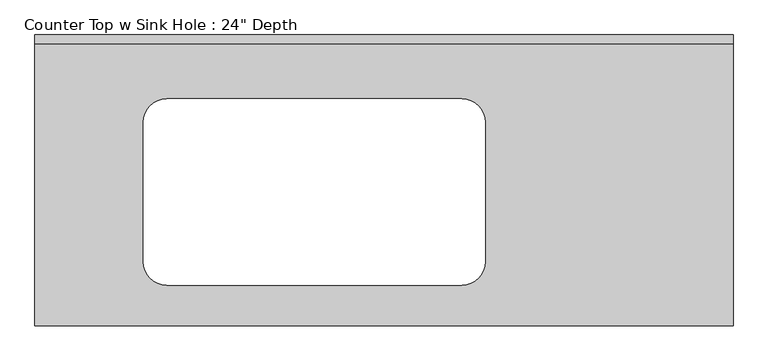
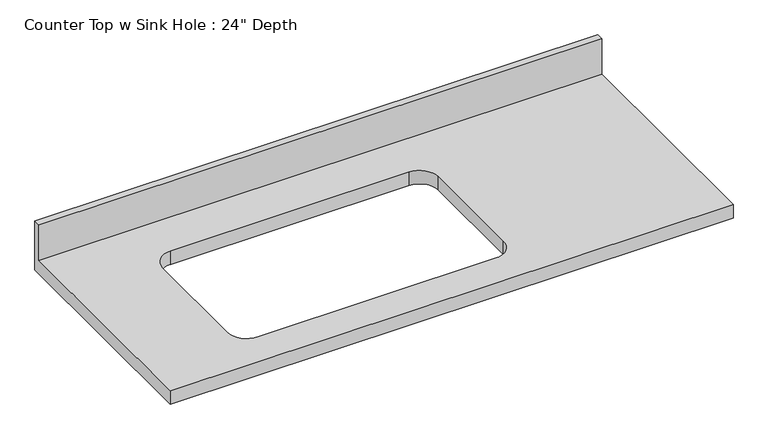
"""IFC4 building model written with IfcOpenShell, lengths in millimetres: furniture geometry."""

from ifc_helpers import new_model, si_unit, frame, origin, place, context, project, spatial, polyline, circle_curve, source, transform, mapped, element, save
from ifc_brep_helpers import plane_surface, revolved_surface, advanced_brep


def furniture_c9930e7d(model_context):
    return source(origin(), model_context, "Body", "AdvancedBrep", [
        advanced_brep(
        [(-1200.4622951, -635.0, 914.4), (323.5377049, -635.0, 914.4), (323.5377049, -19.05, 914.4), (-1200.4622951, -19.05, 914.4), (-913.0885418, -139.7, 914.4), (-268.6360484, -139.7, 914.4), (-217.8360484, -190.5, 914.4), (-217.8360484, -495.3, 914.4), (-268.6360484, -546.1, 914.4), (-913.0885418, -546.1, 914.4), (-963.8885418, -495.3, 914.4), (-963.8885418, -190.5, 914.4), (323.5377049, 0.0, 876.3), (323.5377049, -635.0, 876.3), (-1200.4622951, -635.0, 876.3), (-1200.4622951, 0.0, 876.3), (-268.6360484, -139.7, 876.3), (-913.0885418, -139.7, 876.3), (-963.8885418, -190.5, 876.3), (-963.8885418, -495.3, 876.3), (-913.0885418, -546.1, 876.3), (-268.6360484, -546.1, 876.3), (-217.8360484, -495.3, 876.3), (-217.8360484, -190.5, 876.3), (-1200.4622951, 0.0, 1016.0), (323.5377049, 0.0, 1016.0), (-1200.4622951, -19.05, 1016.0), (323.5377049, -19.05, 1016.0)],
        [
            (0, 1),
            (1, 2),
            (2, 3),
            (3, 0),
            (4, 5),
            (5, 6, circle_curve(frame((-268.6360484, -190.5, 914.4), z_axis=(0.0, 0.0, -1.0), x_axis=(1.0, 0.0, 0.0)), 50.8)),
            (6, 7),
            (7, 8, circle_curve(frame((-268.6360484, -495.3, 914.4), z_axis=(0.0, 0.0, -1.0), x_axis=(1.0, 0.0, 0.0)), 50.8)),
            (8, 9),
            (9, 10, circle_curve(frame((-913.0885418, -495.3, 914.4), z_axis=(0.0, 0.0, -1.0), x_axis=(1.0, 0.0, 0.0)), 50.8)),
            (10, 11),
            (11, 4, circle_curve(frame((-913.0885418, -190.5, 914.4), z_axis=(0.0, 0.0, -1.0), x_axis=(1.0, 0.0, 0.0)), 50.8)),
            (12, 13),
            (13, 14),
            (14, 15),
            (15, 12),
            (16, 17),
            (17, 18, circle_curve(frame((-913.0885418, -190.5, 876.3), z_axis=(0.0, 0.0, 1.0), x_axis=(1.0, 0.0, 0.0)), 50.8)),
            (18, 19),
            (19, 20, circle_curve(frame((-913.0885418, -495.3, 876.3), z_axis=(0.0, 0.0, 1.0), x_axis=(1.0, 0.0, 0.0)), 50.8)),
            (20, 21),
            (21, 22, circle_curve(frame((-268.6360484, -495.3, 876.3), z_axis=(0.0, 0.0, 1.0), x_axis=(1.0, 0.0, 0.0)), 50.8)),
            (22, 23),
            (23, 16, circle_curve(frame((-268.6360484, -190.5, 876.3), z_axis=(0.0, 0.0, 1.0), x_axis=(1.0, 0.0, 0.0)), 50.8)),
            (15, 24),
            (24, 25),
            (25, 12),
            (14, 0),
            (3, 26),
            (26, 24),
            (13, 1),
            (25, 27),
            (27, 2),
            (4, 17),
            (16, 5),
            (11, 18),
            (10, 19),
            (9, 20),
            (8, 21),
            (7, 22),
            (6, 23),
            (26, 27),
        ],
        [
            plane_surface(frame((-1200.4622951, 0.0, 914.4), z_axis=(0.0, 0.0, 1.0), x_axis=(-1.0, 0.0, 0.0))),
            plane_surface(frame((-1200.4622951, 0.0, 876.3), z_axis=(0.0, 0.0, -1.0), x_axis=(1.0, 0.0, 0.0))),
            plane_surface(frame((323.5377049, 0.0, 914.4), z_axis=(0.0, 1.0, 0.0), x_axis=(0.0, 0.0, -1.0))),
            plane_surface(frame((-1200.4622951, 0.0, 914.4), z_axis=(-1.0, 0.0, 0.0), x_axis=(0.0, 0.0, -1.0))),
            plane_surface(frame((-1200.4622951, -635.0, 914.4), z_axis=(0.0, -1.0, 0.0), x_axis=(0.0, 0.0, -1.0))),
            plane_surface(frame((323.5377049, -635.0, 914.4), z_axis=(1.0, 0.0, 0.0), x_axis=(0.0, 0.0, -1.0))),
            plane_surface(frame((-268.6360484, -139.7, 914.4), z_axis=(0.0, -1.0, 0.0), x_axis=(0.0, 0.0, -1.0))),
            revolved_surface(polyline([(-862.2885418000001, -190.5, 914.4), (-862.2885418000001, -190.5, 876.3)]), (-913.0885418, -190.5, 876.3), (0.0, 0.0, 1.0)),
            plane_surface(frame((-963.8885418, -190.5, 914.4), z_axis=(1.0, 0.0, 0.0), x_axis=(0.0, 0.0, -1.0))),
            revolved_surface(polyline([(-862.2885418000001, -495.3, 914.4), (-862.2885418000001, -495.3, 876.3)]), (-913.0885418, -495.3, 876.3), (0.0, 0.0, 1.0)),
            plane_surface(frame((-913.0885418, -546.1, 914.4), z_axis=(0.0, 1.0, 0.0), x_axis=(0.0, 0.0, -1.0))),
            revolved_surface(polyline([(-217.83604839999998, -495.3, 914.4), (-217.83604839999998, -495.3, 876.3)]), (-268.6360484, -495.3, 876.3), (0.0, 0.0, 1.0)),
            plane_surface(frame((-217.8360484, -495.3, 914.4), z_axis=(-1.0, 0.0, 0.0), x_axis=(0.0, 0.0, -1.0))),
            revolved_surface(polyline([(-217.83604839999998, -190.5, 914.4), (-217.83604839999998, -190.5, 876.3)]), (-268.6360484, -190.5, 876.3), (0.0, 0.0, 1.0)),
            plane_surface(frame((-1200.4622951, 0.0, 1016.0), z_axis=(0.0, 0.0, 1.0), x_axis=(0.0, -1.0, 0.0))),
            plane_surface(frame((-1200.4622951, -19.05, 1016.0), z_axis=(0.0, -1.0, 0.0), x_axis=(0.0, 0.0, -1.0))),
        ],
        [
            (0, [[1, 2, 3, 4], [5, 6, 7, 8, 9, 10, 11, 12]]),
            (1, [[13, 14, 15, 16], [17, 18, 19, 20, 21, 22, 23, 24]]),
            (2, [[-16, 25, 26, 27]]),
            (3, [[-15, 28, -4, 29, 30, -25]]),
            (4, [[-1, -28, -14, 31]]),
            (5, [[-13, -27, 32, 33, -2, -31]]),
            (6, [[34, -17, 35, -5]]),
            (7, [[-34, -12, 36, -18]]),
            (8, [[-36, -11, 37, -19]]),
            (9, [[-37, -10, 38, -20]]),
            (10, [[-38, -9, 39, -21]]),
            (11, [[-39, -8, 40, -22]]),
            (12, [[-40, -7, 41, -23]]),
            (13, [[-35, -24, -41, -6]]),
            (14, [[-30, 42, -32, -26]]),
            (15, [[-42, -29, -3, -33]]),
        ],
    ),
    ])


if __name__ == "__main__":
    model = new_model("IFC4")
    model_context = context("Model", 3, world=origin())
    ifc_project = project(units=[si_unit("LENGTHUNIT", "METRE", prefix="MILLI")], contexts=[model_context])
    site = spatial("IfcSite", under=ifc_project)
    building = spatial("IfcBuilding", under=site)
    placement = place(None, origin())
    furniture_shape = furniture_c9930e7d(model_context)
    element("IfcFurniture", 1, ObjectType="Counter Top w Sink Hole : 24\" Depth", at=placement, inside=building, context=model_context, shape_type="MappedRepresentation", body=[
        mapped(furniture_shape, transform((0.0, 0.0, 0.0), x_axis=(1.0, 0.0, 0.0), y_axis=(0.0, 1.0, 0.0), z_axis=(0.0, 0.0, 1.0))),
    ])
    save(model, "model.ifc")

# Revit data of these elements
# Type "Counter Top w Sink Hole : 24\" Depth"
#   Assembly Code = "C1030400"
#   Counter Thickness = 0' - 1 1/2"
#   Depth = 2' - 1"
#   Height = 3' - 0"
#   Length [instance default] = 8' - 0"
#   Sink Location [instance default] = 2' - 0"
#   Sink Location To Wall [instance default] = 0' - 6"
#   Sink Opening Depth [instance default] = 1' - 3"
#   Sink Opening Width [instance default] = 2' - 3"
#   Counter Top Material = none
#   Default Elevation = 0
# Element 1 (IfcFurniture, "Counter Top w Sink Hole : 24\" Depth")
#   Length = 5' - 0"
#   Sink Opening Width = 2' - 4.37215"
#   Materials on its faces: "Counter Top"
# Materials
#   "Counter Top": class "Wood", colour RGB 226 177 128, transparency 0
